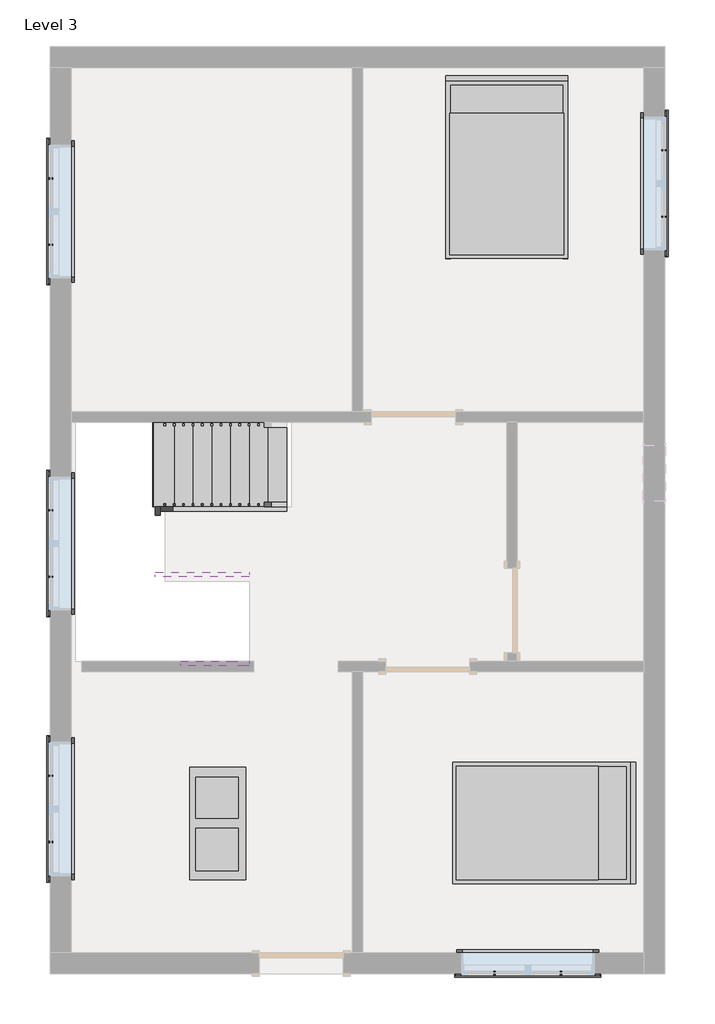
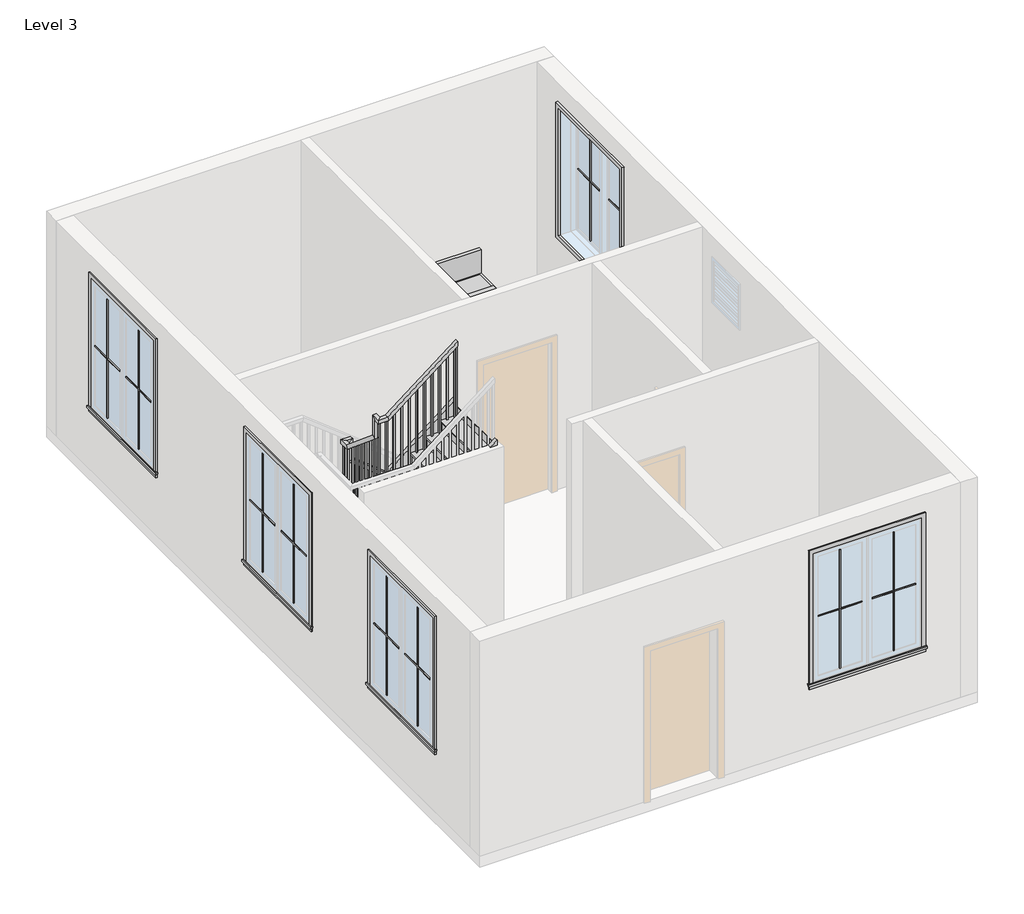
# One storey, part 2 of 2: 21 proxies, 5 members, 2 furniture elements, 1 railing, 1 stair flight.
"""IFC4 building model written with IfcOpenShell, lengths in millimetres."""

from ifc_helpers import new_model, si_unit, frame, origin, place, context, project, spatial, polyline, outline, extrude, faceted_brep, transform, mapped, element, save
from components import muntin_pattern_2x2_muntin_pattern_2x2_bff912c5, muntin_pattern_2x2_muntin_pattern_2x2_c2194282, trim_window_exterior_flat_with_sill_e04b3088, trim_window_interior_flat_picture_frame_2a7685fe, coffee_table_with_brass_mullions_11320_coffee_table_with_5962bef7, bed_17739_bed_17739_15c61121, stair_flight_32cec8f3

model = new_model("IFC4")

# Units and contexts
model_context = context("Model", 3, world=origin())
ifc_project = project(units=[si_unit("LENGTHUNIT", "METRE", prefix="MILLI")], contexts=[model_context])

# Site, building, storey
site = spatial("IfcSite", under=ifc_project)
building = spatial("IfcBuilding", under=site)
storey = spatial("IfcBuildingStorey", under=building, Name="Level 3", Elevation=3200.4)

# Proxies
placement = place(None, origin())
muntin_pattern_2x2_muntin_pattern_2x2_shape = muntin_pattern_2x2_muntin_pattern_2x2_bff912c5(model_context)
element("IfcBuildingElementProxy", 1, Name="Muntin Pattern_2x2 : Muntin Pattern_2x2", ObjectType="Muntin Pattern_2x2 : Muntin Pattern_2x2", at=placement, inside=storey, context=model_context, shape_type="MappedRepresentation", body=[
    mapped(muntin_pattern_2x2_muntin_pattern_2x2_shape, transform((-626.5715247, -5050.1430046, 4184.65), x_axis=(-1.0, 0.0, 0.0), y_axis=(0.0, -1.0, 0.0), z_axis=(0.0, 0.0, 1.0))),
])
element("IfcBuildingElementProxy", 2, Name="Muntin Pattern_2x2 : Muntin Pattern_2x2", ObjectType="Muntin Pattern_2x2 : Muntin Pattern_2x2", at=placement, inside=storey, context=model_context, shape_type="MappedRepresentation", body=[
    mapped(muntin_pattern_2x2_muntin_pattern_2x2_shape, transform((-6159.0090247, -3629.3305046, 4184.65), x_axis=(0.0, 1.0, 0.0), y_axis=(-1.0, 0.0, 0.0), z_axis=(0.0, 0.0, 1.0))),
])
element("IfcBuildingElementProxy", 3, Name="Muntin Pattern_2x2 : Muntin Pattern_2x2", ObjectType="Muntin Pattern_2x2 : Muntin Pattern_2x2", at=placement, inside=storey, context=model_context, shape_type="MappedRepresentation", body=[
    mapped(muntin_pattern_2x2_muntin_pattern_2x2_shape, transform((489.4409753, 3873.1944954, 4184.65), x_axis=(0.0, -1.0, 0.0), y_axis=(1.0, 0.0, 0.0), z_axis=(0.0, 0.0, 1.0))),
])
element("IfcBuildingElementProxy", 4, Name="Muntin Pattern_2x2 : Muntin Pattern_2x2", ObjectType="Muntin Pattern_2x2 : Muntin Pattern_2x2", at=placement, inside=storey, context=model_context, shape_type="MappedRepresentation", body=[
    mapped(muntin_pattern_2x2_muntin_pattern_2x2_shape, transform((-6159.0090247, 2847.6694954, 4184.65), x_axis=(0.0, 1.0, 0.0), y_axis=(-1.0, 0.0, 0.0), z_axis=(0.0, 0.0, 1.0))),
])
element("IfcBuildingElementProxy", 5, Name="Muntin Pattern_2x2 : Muntin Pattern_2x2", ObjectType="Muntin Pattern_2x2 : Muntin Pattern_2x2", at=placement, inside=storey, context=model_context, shape_type="MappedRepresentation", body=[
    mapped(muntin_pattern_2x2_muntin_pattern_2x2_shape, transform((-6159.0090247, -752.7805046, 4184.65), x_axis=(0.0, 1.0, 0.0), y_axis=(-1.0, 0.0, 0.0), z_axis=(0.0, 0.0, 1.0))),
])
muntin_pattern_2x2_muntin_pattern_2x2_2_shape = muntin_pattern_2x2_muntin_pattern_2x2_c2194282(model_context)
element("IfcBuildingElementProxy", 6, Name="Muntin Pattern_2x2 : Muntin Pattern_2x2", ObjectType="Muntin Pattern_2x2 : Muntin Pattern_2x2", at=placement, inside=storey, context=model_context, shape_type="MappedRepresentation", body=[
    mapped(muntin_pattern_2x2_muntin_pattern_2x2_2_shape, transform((-1347.2965247, -5050.1430046, 4184.65), x_axis=(1.0, 0.0, 0.0), y_axis=(0.0, 1.0, 0.0), z_axis=(0.0, 0.0, 1.0))),
])
element("IfcBuildingElementProxy", 7, Name="Muntin Pattern_2x2 : Muntin Pattern_2x2", ObjectType="Muntin Pattern_2x2 : Muntin Pattern_2x2", at=placement, inside=storey, context=model_context, shape_type="MappedRepresentation", body=[
    mapped(muntin_pattern_2x2_muntin_pattern_2x2_2_shape, transform((-6159.0090247, -2908.6055046, 4184.65), x_axis=(0.0, -1.0, 0.0), y_axis=(1.0, 0.0, 0.0), z_axis=(0.0, 0.0, 1.0))),
])
element("IfcBuildingElementProxy", 8, Name="Muntin Pattern_2x2 : Muntin Pattern_2x2", ObjectType="Muntin Pattern_2x2 : Muntin Pattern_2x2", at=placement, inside=storey, context=model_context, shape_type="MappedRepresentation", body=[
    mapped(muntin_pattern_2x2_muntin_pattern_2x2_2_shape, transform((489.4409753, 3152.4694954, 4184.65), x_axis=(0.0, 1.0, 0.0), y_axis=(-1.0, 0.0, 0.0), z_axis=(0.0, 0.0, 1.0))),
])
element("IfcBuildingElementProxy", 9, Name="Muntin Pattern_2x2 : Muntin Pattern_2x2", ObjectType="Muntin Pattern_2x2 : Muntin Pattern_2x2", at=placement, inside=storey, context=model_context, shape_type="MappedRepresentation", body=[
    mapped(muntin_pattern_2x2_muntin_pattern_2x2_2_shape, transform((-6159.0090247, 3568.3944954, 4184.65), x_axis=(0.0, -1.0, 0.0), y_axis=(1.0, 0.0, 0.0), z_axis=(0.0, 0.0, 1.0))),
])
element("IfcBuildingElementProxy", 10, Name="Muntin Pattern_2x2 : Muntin Pattern_2x2", ObjectType="Muntin Pattern_2x2 : Muntin Pattern_2x2", at=placement, inside=storey, context=model_context, shape_type="MappedRepresentation", body=[
    mapped(muntin_pattern_2x2_muntin_pattern_2x2_2_shape, transform((-6159.0090247, -32.0555046, 4184.65), x_axis=(0.0, -1.0, 0.0), y_axis=(1.0, 0.0, 0.0), z_axis=(0.0, 0.0, 1.0))),
])
trim_window_exterior_flat_with_sill_shape = trim_window_exterior_flat_with_sill_e04b3088(model_context)
element("IfcBuildingElementProxy", 11, Name="Trim-Window-Exterior-Flat : with Sill", ObjectType="Trim-Window-Exterior-Flat : with Sill", at=placement, inside=storey, context=model_context, shape_type="MappedRepresentation", body=[
    mapped(trim_window_exterior_flat_with_sill_shape, transform((-986.9340247, -5059.6680046, 5943.6), x_axis=(1.0, 0.0, 0.0), y_axis=(0.0, 0.0, 1.0), z_axis=(0.0, -1.0, 0.0))),
])
element("IfcBuildingElementProxy", 12, Name="Trim-Window-Exterior-Flat : with Sill", ObjectType="Trim-Window-Exterior-Flat : with Sill", at=placement, inside=storey, context=model_context, shape_type="MappedRepresentation", body=[
    mapped(trim_window_exterior_flat_with_sill_shape, transform((-6168.5340247, -3268.9680046, 5943.6), x_axis=(0.0, -1.0, 0.0), y_axis=(0.0, 0.0, 1.0), z_axis=(-1.0, 0.0, 0.0))),
])
element("IfcBuildingElementProxy", 13, Name="Trim-Window-Exterior-Flat : with Sill", ObjectType="Trim-Window-Exterior-Flat : with Sill", at=placement, inside=storey, context=model_context, shape_type="MappedRepresentation", body=[
    mapped(trim_window_exterior_flat_with_sill_shape, transform((498.9659753, 3512.8319954, 5943.6), x_axis=(0.0, 1.0, 0.0), y_axis=(0.0, 0.0, 1.0), z_axis=(1.0, 0.0, 0.0))),
])
element("IfcBuildingElementProxy", 14, Name="Trim-Window-Exterior-Flat : with Sill", ObjectType="Trim-Window-Exterior-Flat : with Sill", at=placement, inside=storey, context=model_context, shape_type="MappedRepresentation", body=[
    mapped(trim_window_exterior_flat_with_sill_shape, transform((-6168.5340247, 3208.0319954, 5943.6), x_axis=(0.0, -1.0, 0.0), y_axis=(0.0, 0.0, 1.0), z_axis=(-1.0, 0.0, 0.0))),
])
element("IfcBuildingElementProxy", 15, Name="Trim-Window-Exterior-Flat : with Sill", ObjectType="Trim-Window-Exterior-Flat : with Sill", at=placement, inside=storey, context=model_context, shape_type="MappedRepresentation", body=[
    mapped(trim_window_exterior_flat_with_sill_shape, transform((-6168.5340247, -392.4180046, 5943.6), x_axis=(0.0, -1.0, 0.0), y_axis=(0.0, 0.0, 1.0), z_axis=(-1.0, 0.0, 0.0))),
])
trim_window_interior_flat_picture_frame_shape = trim_window_interior_flat_picture_frame_2a7685fe(model_context)
element("IfcBuildingElementProxy", 16, Name="Trim-Window-Interior-Flat : Picture Frame", ObjectType="Trim-Window-Interior-Flat : Picture Frame", at=placement, inside=storey, context=model_context, shape_type="MappedRepresentation", body=[
    mapped(trim_window_interior_flat_picture_frame_shape, transform((-986.9340247, -4831.0680046, 5943.6), x_axis=(-1.0, 0.0, 0.0), y_axis=(0.0, 0.0, 1.0), z_axis=(0.0, 1.0, 0.0))),
])
element("IfcBuildingElementProxy", 17, Name="Trim-Window-Interior-Flat : Picture Frame", ObjectType="Trim-Window-Interior-Flat : Picture Frame", at=placement, inside=storey, context=model_context, shape_type="MappedRepresentation", body=[
    mapped(trim_window_interior_flat_picture_frame_shape, transform((-5939.9340247, -3268.9680046, 5943.6), x_axis=(0.0, 1.0, 0.0), y_axis=(0.0, 0.0, 1.0), z_axis=(1.0, 0.0, 0.0))),
])
element("IfcBuildingElementProxy", 18, Name="Trim-Window-Interior-Flat : Picture Frame", ObjectType="Trim-Window-Interior-Flat : Picture Frame", at=placement, inside=storey, context=model_context, shape_type="MappedRepresentation", body=[
    mapped(trim_window_interior_flat_picture_frame_shape, transform((270.3659753, 3512.8319954, 5943.6), x_axis=(0.0, -1.0, 0.0), y_axis=(0.0, 0.0, 1.0), z_axis=(-1.0, 0.0, 0.0))),
])
element("IfcBuildingElementProxy", 19, Name="Trim-Window-Interior-Flat : Picture Frame", ObjectType="Trim-Window-Interior-Flat : Picture Frame", at=placement, inside=storey, context=model_context, shape_type="MappedRepresentation", body=[
    mapped(trim_window_interior_flat_picture_frame_shape, transform((-5939.9340247, 3208.0319954, 5943.6), x_axis=(0.0, 1.0, 0.0), y_axis=(0.0, 0.0, 1.0), z_axis=(1.0, 0.0, 0.0))),
])
element("IfcBuildingElementProxy", 20, Name="Trim-Window-Interior-Flat : Picture Frame", ObjectType="Trim-Window-Interior-Flat : Picture Frame", at=placement, inside=storey, context=model_context, shape_type="MappedRepresentation", body=[
    mapped(trim_window_interior_flat_picture_frame_shape, transform((-5939.9340247, -392.4180046, 5943.6), x_axis=(0.0, 1.0, 0.0), y_axis=(0.0, 0.0, 1.0), z_axis=(1.0, 0.0, 0.0))),
])
coffee_table_with_brass_mullions_11320_coffee_table_with_shape = coffee_table_with_brass_mullions_11320_coffee_table_with_5962bef7(model_context)
element("IfcBuildingElementProxy", 21, Name="coffee_table_with_brass_mullions_11320 : coffee_table_with_brass_mullions_11320", ObjectType="coffee_table_with_brass_mullions_11320 : coffee_table_with_brass_mullions_11320", at=placement, inside=storey, context=model_context, shape_type="MappedRepresentation", body=[
    mapped(coffee_table_with_brass_mullions_11320_coffee_table_with_shape, transform((-3920.6340247, -2792.7180046, 3200.4), x_axis=(0.0, 1.0, 0.0), y_axis=(-1.0, 0.0, 0.0), z_axis=(0.0, 0.0, 1.0))),
])

# Furniture
bed_17739_bed_17739_shape = bed_17739_bed_17739_15c61121(model_context)
element("IfcFurniture", 22, ObjectType="Bed_17739 : Bed_17739", at=placement, inside=storey, context=model_context, shape_type="MappedRepresentation", body=[
    mapped(bed_17739_bed_17739_shape, transform((-1215.5340247, 3665.2319954, 3200.4), x_axis=(1.0, 0.0, 0.0), y_axis=(0.0, 1.0, 0.0), z_axis=(0.0, 0.0, 1.0))),
])
element("IfcFurniture", 23, ObjectType="Bed_17739 : Bed_17739", at=placement, inside=storey, context=model_context, shape_type="MappedRepresentation", body=[
    mapped(bed_17739_bed_17739_shape, transform((-834.5340247, -3421.3680046, 3200.4), x_axis=(0.0, -1.0, 0.0), y_axis=(1.0, 0.0, 0.0), z_axis=(0.0, 0.0, 1.0))),
])

# Members
element("IfcMember", 24, ObjectType="Stringer - 2\" Width", at=placement, inside=storey, context=model_context, shape_type="SweptSolid", body=[
    extrude(outline(polyline([(3200.4, -3603.1340247), (3431.9686588, -3603.1340247), (4514.8107641, -4974.7340247), (4126.4725136, -4974.7340247), (3200.4, -3801.7088408), (3200.4, -3603.1340247)])), frame((0.0, -43.1680046, 0.0), z_axis=(0.0, 1.0, 0.0), x_axis=(0.0, 0.0, 1.0)), (0.0, 0.0, 1.0), 50.8),
])
element("IfcMember", 25, ObjectType="Stringer - 2\" Width", at=placement, inside=storey, context=model_context, shape_type="SweptSolid", body=[
    extrude(outline(polyline([(7.6319954, 4721.6930346), (7.6319954, 4323.2154064), (-703.5680046, 4922.1206696), (-703.5680046, 5320.5982978), (7.6319954, 4721.6930346)])), frame((-5025.5340247, 0.0, 0.0), z_axis=(1.0, 0.0, 0.0), x_axis=(0.0, 1.0, 0.0)), (0.0, 0.0, 1.0), 50.8),
])
element("IfcMember", 26, ObjectType="Stringer - 2\" Width", at=placement, inside=storey, context=model_context, shape_type="SweptSolid", body=[
    extrude(outline(polyline([(5517.442343, -5025.5340247), (5129.1040926, -5025.5340247), (5931.2093557, -4009.5340247), (6319.5476062, -4009.5340247), (5517.442343, -5025.5340247)])), frame((0.0, -754.3680046, 0.0), z_axis=(0.0, 1.0, 0.0), x_axis=(0.0, 0.0, 1.0)), (0.0, 0.0, 1.0), 50.8),
])
element("IfcMember", 27, ObjectType="Stringer - 2\" Width", at=placement, inside=storey, context=model_context, shape_type="SweptSolid", body=[
    extrude(outline(polyline([(3200.4, -3603.1340247), (3431.9686588, -3603.1340247), (3951.671982, -4261.4249007), (3951.671982, -4753.3200179), (3200.4, -3801.7088408), (3200.4, -3603.1340247)])), frame((0.0, 922.0319954, 0.0), z_axis=(0.0, 1.0, 0.0), x_axis=(0.0, 0.0, 1.0)), (0.0, 0.0, 1.0), 50.8),
])
element("IfcMember", 28, ObjectType="Stringer - 2\" Width", at=placement, inside=storey, context=model_context, shape_type="SweptSolid", body=[
    extrude(outline(polyline([(5734.9206696, -4258.1663605), (5931.2093557, -4009.5340247), (6319.5476062, -4009.5340247), (5734.9206696, -4750.0614777), (5734.9206696, -4258.1663605)])), frame((0.0, -1719.5680046, 0.0), z_axis=(0.0, 1.0, 0.0), x_axis=(0.0, 0.0, 1.0)), (0.0, 0.0, 1.0), 50.8),
])

# Railing
element("IfcRailing", 29, ObjectType="Handrail - Rectangular", at=placement, inside=storey, context=model_context, shape_type="SolidModel", body=[
    faceted_brep([(-3603.1340247, 7.6319954, 4275.2210526), (-3603.1340247, 7.6319954, 4210.4980109), (-3603.1340247, 58.4319954, 4210.4980109), (-3603.1340247, 58.4319954, 4275.2210526), (-4949.3340247, 7.6319954, 5338.0105263), (-5000.1340247, 7.6319954, 5313.3927477), (-5000.1340247, 58.4319954, 5313.3927477), (-4949.3340247, 58.4319954, 5338.0105263), (-4949.3340247, 7.6319954, 5622.7578947), (-5000.1340247, 7.6319954, 5571.9578947), (-5000.1340247, 58.4319954, 5571.9578947), (-4949.3340247, 58.4319954, 5622.7578947), (-5025.5340247, 7.6319954, 5622.7578947), (-5025.5340247, 7.6319954, 5571.9578947), (-5076.3340247, 58.4319954, 5571.9578947), (-5076.3340247, 58.4319954, 5622.7578947), (-5025.5340247, -68.5680046, 5622.7578947), (-5025.5340247, -87.1083685, 5571.9578947), (-5076.3340247, -87.1083685, 5571.9578947), (-5076.3340247, -68.5680046, 5622.7578947), (-5025.5340247, -678.1680046, 6136.1052632), (-5025.5340247, -728.9680046, 6112.4712725), (-5076.3340247, -728.9680046, 6112.4712725), (-5076.3340247, -678.1680046, 6136.1052632), (-5025.5340247, -678.1680046, 6420.8526316), (-5025.5340247, -728.9680046, 6370.0526316), (-5076.3340247, -728.9680046, 6370.0526316), (-5076.3340247, -678.1680046, 6420.8526316), (-5025.5340247, -754.3680046, 6420.8526316), (-5025.5340247, -754.3680046, 6370.0526316), (-5076.3340247, -805.1680046, 6370.0526316), (-5076.3340247, -805.1680046, 6420.8526316), (-4949.3340247, -754.3680046, 6420.8526316), (-4931.6981718, -754.3680046, 6370.0526316), (-4931.6981718, -805.1680046, 6370.0526316), (-4949.3340247, -805.1680046, 6420.8526316), (-4009.5340247, -754.3680046, 7162.8), (-4009.5340247, -805.1680046, 7162.8), (-4009.5340247, -805.1680046, 7098.0769583), (-4009.5340247, -754.3680046, 7098.0769583)], [[[0, 1, 2, 3]], [[1, 0, 4, 5]], [[2, 1, 5, 6]], [[3, 2, 6, 7]], [[0, 3, 7, 4]], [[5, 4, 8, 9]], [[6, 5, 9, 10]], [[7, 6, 10, 11]], [[4, 7, 11, 8]], [[9, 8, 12, 13]], [[10, 9, 13, 14]], [[11, 10, 14, 15]], [[8, 11, 15, 12]], [[13, 12, 16, 17]], [[14, 13, 17, 18]], [[15, 14, 18, 19]], [[12, 15, 19, 16]], [[17, 16, 20, 21]], [[18, 17, 21, 22]], [[19, 18, 22, 23]], [[16, 19, 23, 20]], [[21, 20, 24, 25]], [[22, 21, 25, 26]], [[23, 22, 26, 27]], [[20, 23, 27, 24]], [[25, 24, 28, 29]], [[26, 25, 29, 30]], [[27, 26, 30, 31]], [[24, 27, 31, 28]], [[29, 28, 32, 33]], [[30, 29, 33, 34]], [[31, 30, 34, 35]], [[28, 31, 35, 32]], [[36, 37, 38, 39]], [[33, 32, 36, 39]], [[34, 33, 39, 38]], [[35, 34, 38, 37]], [[32, 35, 37, 36]]]),
    extrude(outline(polyline([(7070.5045898, -4044.4590247), (6087.9789474, -4044.4590247), (6087.9789474, -4025.4090247), (7085.5440635, -4025.4090247), (7070.5045898, -4044.4590247)])), frame((0.0, -789.2930046, 0.0), z_axis=(0.0, 1.0, 0.0), x_axis=(0.0, 0.0, 1.0)), (0.0, 0.0, 1.0), 19.05),
    extrude(outline(polyline([(6990.2940635, -4146.0590247), (6087.9789474, -4146.0590247), (6087.9789474, -4127.0090247), (7005.3335372, -4127.0090247), (6990.2940635, -4146.0590247)])), frame((0.0, -789.2930046, 0.0), z_axis=(0.0, 1.0, 0.0), x_axis=(0.0, 0.0, 1.0)), (0.0, 0.0, 1.0), 19.05),
    extrude(outline(polyline([(6910.0835372, -4247.6590247), (5927.5578947, -4247.6590247), (5927.5578947, -4228.6090247), (6925.1230109, -4228.6090247), (6910.0835372, -4247.6590247)])), frame((0.0, -789.2930046, 0.0), z_axis=(0.0, 1.0, 0.0), x_axis=(0.0, 0.0, 1.0)), (0.0, 0.0, 1.0), 19.05),
    extrude(outline(polyline([(6829.8730109, -4349.2590247), (5927.5578947, -4349.2590247), (5927.5578947, -4330.2090247), (6844.9124846, -4330.2090247), (6829.8730109, -4349.2590247)])), frame((0.0, -789.2930046, 0.0), z_axis=(0.0, 1.0, 0.0), x_axis=(0.0, 0.0, 1.0)), (0.0, 0.0, 1.0), 19.05),
    extrude(outline(polyline([(6749.6624846, -4450.8590247), (5767.1368421, -4450.8590247), (5767.1368421, -4431.8090247), (6764.7019583, -4431.8090247), (6749.6624846, -4450.8590247)])), frame((0.0, -789.2930046, 0.0), z_axis=(0.0, 1.0, 0.0), x_axis=(0.0, 0.0, 1.0)), (0.0, 0.0, 1.0), 19.05),
    extrude(outline(polyline([(6669.4519583, -4552.4590247), (5767.1368421, -4552.4590247), (5767.1368421, -4533.4090247), (6684.4914319, -4533.4090247), (6669.4519583, -4552.4590247)])), frame((0.0, -789.2930046, 0.0), z_axis=(0.0, 1.0, 0.0), x_axis=(0.0, 0.0, 1.0)), (0.0, 0.0, 1.0), 19.05),
    extrude(outline(polyline([(6589.2414319, -4654.0590247), (5606.7157895, -4654.0590247), (5606.7157895, -4635.0090247), (6604.2809056, -4635.0090247), (6589.2414319, -4654.0590247)])), frame((0.0, -789.2930046, 0.0), z_axis=(0.0, 1.0, 0.0), x_axis=(0.0, 0.0, 1.0)), (0.0, 0.0, 1.0), 19.05),
    extrude(outline(polyline([(6509.0309056, -4755.6590247), (5606.7157895, -4755.6590247), (5606.7157895, -4736.6090247), (6524.0703793, -4736.6090247), (6509.0309056, -4755.6590247)])), frame((0.0, -789.2930046, 0.0), z_axis=(0.0, 1.0, 0.0), x_axis=(0.0, 0.0, 1.0)), (0.0, 0.0, 1.0), 19.05),
    extrude(outline(polyline([(6428.8203793, -4857.2590247), (5446.2947368, -4857.2590247), (5446.2947368, -4838.2090247), (6443.859853, -4838.2090247), (6428.8203793, -4857.2590247)])), frame((0.0, -789.2930046, 0.0), z_axis=(0.0, 1.0, 0.0), x_axis=(0.0, 0.0, 1.0)), (0.0, 0.0, 1.0), 19.05),
    extrude(outline(polyline([(6348.609853, -4958.8590247), (5446.2947368, -4958.8590247), (5446.2947368, -4939.8090247), (6363.6493267, -4939.8090247), (6348.609853, -4958.8590247)])), frame((0.0, -789.2930046, 0.0), z_axis=(0.0, 1.0, 0.0), x_axis=(0.0, 0.0, 1.0)), (0.0, 0.0, 1.0), 19.05),
    extrude(outline(polyline([(-668.6430046, 6061.6712725), (-668.6430046, 5125.4526316), (-687.6930046, 5125.4526316), (-687.6930046, 6077.7133778), (-668.6430046, 6061.6712725)])), frame((-5060.4590247, 0.0, 0.0), z_axis=(1.0, 0.0, 0.0), x_axis=(0.0, 1.0, 0.0)), (0.0, 0.0, 1.0), 19.05),
    extrude(outline(polyline([(-567.0430046, 5976.1133778), (-567.0430046, 5125.4526316), (-586.0930046, 5125.4526316), (-586.0930046, 5992.155483), (-567.0430046, 5976.1133778)])), frame((-5060.4590247, 0.0, 0.0), z_axis=(1.0, 0.0, 0.0), x_axis=(0.0, 1.0, 0.0)), (0.0, 0.0, 1.0), 19.05),
    extrude(outline(polyline([(-465.4430046, 5890.555483), (-465.4430046, 4965.0315789), (-484.4930046, 4965.0315789), (-484.4930046, 5906.5975883), (-465.4430046, 5890.555483)])), frame((-5060.4590247, 0.0, 0.0), z_axis=(1.0, 0.0, 0.0), x_axis=(0.0, 1.0, 0.0)), (0.0, 0.0, 1.0), 19.05),
    extrude(outline(polyline([(-363.8430046, 5804.9975883), (-363.8430046, 4965.0315789), (-382.8930046, 4965.0315789), (-382.8930046, 5821.0396935), (-363.8430046, 5804.9975883)])), frame((-5060.4590247, 0.0, 0.0), z_axis=(1.0, 0.0, 0.0), x_axis=(0.0, 1.0, 0.0)), (0.0, 0.0, 1.0), 19.05),
    extrude(outline(polyline([(-262.2430046, 5719.4396935), (-262.2430046, 4804.6105263), (-281.2930046, 4804.6105263), (-281.2930046, 5735.4817988), (-262.2430046, 5719.4396935)])), frame((-5060.4590247, 0.0, 0.0), z_axis=(1.0, 0.0, 0.0), x_axis=(0.0, 1.0, 0.0)), (0.0, 0.0, 1.0), 19.05),
    extrude(outline(polyline([(-160.6430046, 5633.8817988), (-160.6430046, 4804.6105263), (-179.6930046, 4804.6105263), (-179.6930046, 5649.9239041), (-160.6430046, 5633.8817988)])), frame((-5060.4590247, 0.0, 0.0), z_axis=(1.0, 0.0, 0.0), x_axis=(0.0, 1.0, 0.0)), (0.0, 0.0, 1.0), 19.05),
    extrude(outline(polyline([(-59.0430046, 5548.3239041), (-59.0430046, 4644.1894737), (-78.0930046, 4644.1894737), (-78.0930046, 5564.3660093), (-59.0430046, 5548.3239041)])), frame((-5060.4590247, 0.0, 0.0), z_axis=(1.0, 0.0, 0.0), x_axis=(0.0, 1.0, 0.0)), (0.0, 0.0, 1.0), 19.05),
    extrude(outline(polyline([(-5016.0090247, 23.5069954), (-5035.0590247, 23.5069954), (-5035.0590247, 42.5569954), (-5016.0090247, 42.5569954), (-5016.0090247, 23.5069954)])), frame((0.0, 0.0, 4483.7684211), z_axis=(0.0, 0.0, 1.0), x_axis=(1.0, 0.0, 0.0)), (0.0, 0.0, 1.0), 1088.1894737),
    extrude(outline(polyline([(5260.7545898, -4933.4590247), (4323.3473684, -4933.4590247), (4323.3473684, -4914.4090247), (5245.7151161, -4914.4090247), (5260.7545898, -4933.4590247)])), frame((0.0, 23.5069954, 0.0), z_axis=(0.0, 1.0, 0.0), x_axis=(0.0, 0.0, 1.0)), (0.0, 0.0, 1.0), 19.05),
    extrude(outline(polyline([(5180.5440635, -4831.8590247), (4323.3473684, -4831.8590247), (4323.3473684, -4812.8090247), (5165.5045898, -4812.8090247), (5180.5440635, -4831.8590247)])), frame((0.0, 23.5069954, 0.0), z_axis=(0.0, 1.0, 0.0), x_axis=(0.0, 0.0, 1.0)), (0.0, 0.0, 1.0), 19.05),
    extrude(outline(polyline([(5100.3335372, -4730.2590247), (4162.9263158, -4730.2590247), (4162.9263158, -4711.2090247), (5085.2940635, -4711.2090247), (5100.3335372, -4730.2590247)])), frame((0.0, 23.5069954, 0.0), z_axis=(0.0, 1.0, 0.0), x_axis=(0.0, 0.0, 1.0)), (0.0, 0.0, 1.0), 19.05),
    extrude(outline(polyline([(5020.1230109, -4628.6590247), (4162.9263158, -4628.6590247), (4162.9263158, -4609.6090247), (5005.0835372, -4609.6090247), (5020.1230109, -4628.6590247)])), frame((0.0, 23.5069954, 0.0), z_axis=(0.0, 1.0, 0.0), x_axis=(0.0, 0.0, 1.0)), (0.0, 0.0, 1.0), 19.05),
    extrude(outline(polyline([(4939.9124846, -4527.0590247), (4002.5052632, -4527.0590247), (4002.5052632, -4508.0090247), (4924.8730109, -4508.0090247), (4939.9124846, -4527.0590247)])), frame((0.0, 23.5069954, 0.0), z_axis=(0.0, 1.0, 0.0), x_axis=(0.0, 0.0, 1.0)), (0.0, 0.0, 1.0), 19.05),
    extrude(outline(polyline([(4859.7019583, -4425.4590247), (4002.5052632, -4425.4590247), (4002.5052632, -4406.4090247), (4844.6624846, -4406.4090247), (4859.7019583, -4425.4590247)])), frame((0.0, 23.5069954, 0.0), z_axis=(0.0, 1.0, 0.0), x_axis=(0.0, 0.0, 1.0)), (0.0, 0.0, 1.0), 19.05),
    extrude(outline(polyline([(4779.4914319, -4323.8590247), (3842.0842105, -4323.8590247), (3842.0842105, -4304.8090247), (4764.4519583, -4304.8090247), (4779.4914319, -4323.8590247)])), frame((0.0, 23.5069954, 0.0), z_axis=(0.0, 1.0, 0.0), x_axis=(0.0, 0.0, 1.0)), (0.0, 0.0, 1.0), 19.05),
    extrude(outline(polyline([(4699.2809056, -4222.2590247), (3842.0842105, -4222.2590247), (3842.0842105, -4203.2090247), (4684.2414319, -4203.2090247), (4699.2809056, -4222.2590247)])), frame((0.0, 23.5069954, 0.0), z_axis=(0.0, 1.0, 0.0), x_axis=(0.0, 0.0, 1.0)), (0.0, 0.0, 1.0), 19.05),
    extrude(outline(polyline([(4619.0703793, -4120.6590247), (3681.6631579, -4120.6590247), (3681.6631579, -4101.6090247), (4604.0309056, -4101.6090247), (4619.0703793, -4120.6590247)])), frame((0.0, 23.5069954, 0.0), z_axis=(0.0, 1.0, 0.0), x_axis=(0.0, 0.0, 1.0)), (0.0, 0.0, 1.0), 19.05),
    extrude(outline(polyline([(4538.859853, -4019.0590247), (3681.6631579, -4019.0590247), (3681.6631579, -4000.0090247), (4523.8203793, -4000.0090247), (4538.859853, -4019.0590247)])), frame((0.0, 23.5069954, 0.0), z_axis=(0.0, 1.0, 0.0), x_axis=(0.0, 0.0, 1.0)), (0.0, 0.0, 1.0), 19.05),
    extrude(outline(polyline([(4458.6493267, -3917.4590247), (3521.2421053, -3917.4590247), (3521.2421053, -3898.4090247), (4443.609853, -3898.4090247), (4458.6493267, -3917.4590247)])), frame((0.0, 23.5069954, 0.0), z_axis=(0.0, 1.0, 0.0), x_axis=(0.0, 0.0, 1.0)), (0.0, 0.0, 1.0), 19.05),
    extrude(outline(polyline([(4378.4388004, -3815.8590247), (3521.2421053, -3815.8590247), (3521.2421053, -3796.8090247), (4363.3993267, -3796.8090247), (4378.4388004, -3815.8590247)])), frame((0.0, 23.5069954, 0.0), z_axis=(0.0, 1.0, 0.0), x_axis=(0.0, 0.0, 1.0)), (0.0, 0.0, 1.0), 19.05),
    extrude(outline(polyline([(4298.228274, -3714.2590247), (3360.8210526, -3714.2590247), (3360.8210526, -3695.2090247), (4283.1888004, -3695.2090247), (4298.228274, -3714.2590247)])), frame((0.0, 23.5069954, 0.0), z_axis=(0.0, 1.0, 0.0), x_axis=(0.0, 0.0, 1.0)), (0.0, 0.0, 1.0), 19.05),
    extrude(outline(polyline([(-5041.4090247, -770.2430046), (-5041.4090247, -789.2930046), (-5060.4590247, -789.2930046), (-5060.4590247, -770.2430046), (-5041.4090247, -770.2430046)])), frame((0.0, 0.0, 5285.8736842), z_axis=(0.0, 0.0, 1.0), x_axis=(1.0, 0.0, 0.0)), (0.0, 0.0, 1.0), 1084.1789474),
    extrude(outline(polyline([(-5041.4090247, 23.5069954), (-5060.4590247, 23.5069954), (-5060.4590247, 42.5569954), (-5041.4090247, 42.5569954), (-5041.4090247, 23.5069954)])), frame((0.0, 0.0, 4483.7684211), z_axis=(0.0, 0.0, 1.0), x_axis=(1.0, 0.0, 0.0)), (0.0, 0.0, 1.0), 1088.1894737),
    extrude(outline(polyline([(7083.0374846, -4028.5840247), (6087.9789474, -4028.5840247), (6087.9789474, -4009.5340247), (7098.0769583, -4009.5340247), (7083.0374846, -4028.5840247)])), frame((0.0, -789.2930046, 0.0), z_axis=(0.0, 1.0, 0.0), x_axis=(0.0, 0.0, 1.0)), (0.0, 0.0, 1.0), 19.05),
    extrude(outline(polyline([(4225.5374846, -3622.1840247), (3360.8210526, -3622.1840247), (3360.8210526, -3603.1340247), (4210.4980109, -3603.1340247), (4225.5374846, -3622.1840247)])), frame((0.0, 23.5069954, 0.0), z_axis=(0.0, 1.0, 0.0), x_axis=(0.0, 0.0, 1.0)), (0.0, 0.0, 1.0), 19.05),
])

# Stair flight
stair_flight_shape = stair_flight_32cec8f3(model_context)
element("IfcStairFlight", 30, ObjectType="2\" Tread 1\" Nosing 1/4\" Riser", at=placement, inside=storey, context=model_context, shape_type="MappedRepresentation", body=[
    mapped(stair_flight_shape, transform((0.0, 0.0, 0.0), x_axis=(1.0, 0.0, 0.0), y_axis=(0.0, 1.0, 0.0), z_axis=(0.0, 0.0, 1.0))),
])

save(model, "model.ifc")

# Revit data of these elements
# Type "Muntin Pattern_2x2 : Muntin Pattern_2x2"
#   Width [instance default] = 4' - 0"
#   Thickness = 0' - 0 1/2"
#   Height [instance default] = 4' - 0"
#   Distance = 0' - 0 3/4"
#   Interior Material [instance default] = none
#   Exterior Material [instance default] = none
#   Default Elevation = 0
# Type "Trim-Window-Exterior-Flat : with Sill"
#   Trim Width = 0' - 2 1/4"
#   Trim Thickness_Picture Frame = 0' - 1 1/4"
#   Trim Thickness_with Sill = 0' - 0 3/4"
#   Sill Thickness = 0' - 1 1/4"
#   Opening Width [instance default] = 2' - 0"
#   Opening Height [instance default] = 3' - 0"
#   Default Elevation = 4' - 0"
#   Sill = yes
#   Picture Frame = no
#   Trim Material [instance default] = none
# Type "Trim-Window-Interior-Flat : Picture Frame"
#   Trim Thickness_Picture Frame = 0' - 1 1/4"
#   Trim Width = 0' - 2 1/4"
#   Trim Thickness_with Sill = 0' - 0 3/4"
#   Sill Thickness = 0' - 1 1/4"
#   Opening Width [instance default] = 2' - 0"
#   Opening Height [instance default] = 3' - 0"
#   Default Elevation = 4' - 0"
#   Sill = no
#   Picture Frame = yes
#   Trim Material [instance default] = none
# Type "coffee_table_with_brass_mullions_11320 : coffee_table_with_brass_mullions_11320"
#   Default Elevation = 0
# Type "Bed_17739 : Bed_17739"
#   Default Elevation = 0
# Type "Handrail - Rectangular"
#   Assembly Code = "C2010400"
#   built-in parameter 1008612 = 0.0416667 (stored number, unit not read)
#   built-in parameter 1008611 = 0.0416667 (stored number, unit not read)
#   built-in parameter 1008609 = 0.333333 (stored number, unit not read)
#   built-in parameter 1008604 = 0.166667 (stored number, unit not read)
#   built-in parameter 1008603 = 0.166667 (stored number, unit not read)
#   Railing Height = 3' - 0"
#   built-in parameter 1008630 = 2
#   built-in parameter 1008610 = 2
#   built-in parameter 1008618 = Baluster - Square : 3/4"
# Elements 1, 2, 3, 4, 5, 6, 7, 8, 9, 10 (IfcBuildingElementProxy, "Muntin Pattern_2x2 : Muntin Pattern_2x2")
#   Width = 1' - 11 1/8"
#   Height = 5' - 6 1/2"
#   Interior Material = Wood - Stained
#   Exterior Material = Clad - White
#   Phase Created = New Construction
#   Materials on its faces: "Clad - White", "Wood - Stained"
# Elements 11, 12, 13, 14, 15 (IfcBuildingElementProxy, "Trim-Window-Exterior-Flat : with Sill")
#   Opening Width = 4' - 9"
#   Opening Height = 6' - 0"
#   Trim Material = Clad - White
#   Phase Created = New Construction
#   Materials on its faces: "Clad - White"
# Elements 16, 17, 18, 19, 20 (IfcBuildingElementProxy, "Trim-Window-Interior-Flat : Picture Frame")
#   Opening Width = 4' - 9"
#   Opening Height = 6' - 0"
#   Trim Material = Wood - Stained
#   Phase Created = New Construction
#   Materials on its faces: "Wood - Stained"
# Element 21 (IfcBuildingElementProxy, "coffee_table_with_brass_mullions_11320 : coffee_table_with_brass_mullions_11320")
#   Phase Created = New Construction
#   Materials on its faces: "Default Wall", "TABLE", "Glass", "Default"
# Elements 22, 23 (IfcFurniture, "Bed_17739 : Bed_17739")
#   Phase Created = New Construction
#   Materials on its faces: "legs", "sheets", "bed frame", "Blanket"
# Elements 24, 25, 26, 27, 28 (IfcMember, "Stringer - 2\" Width")
#   Phase Created = New Construction
# Element 29 (IfcRailing, "Handrail - Rectangular")
#   Phase Created = New Construction
#   Materials on its faces: "Oak Flooring"
# Element 30 (IfcStairFlight, "2\" Tread 1\" Nosing 1/4\" Riser")
#   Phase Created = New Construction
# Materials
#   "Clad - White": class "Wood", colour RGB 242 242 238, transparency 0, Cost = 0
#   "Wood - Stained": class "Wood", colour RGB 224 178 126, transparency 0, Cost = 0
#   "Default Wall": colour RGB 128 128 128, transparency 0, Cost = 0
#   "TABLE": class "Generic", colour RGB 120 120 120, transparency 0, Cost = 0
#   "Glass": class "Glass", colour RGB 0 128 192, transparency 0.75, Description = "Soda Lime Glass", Cost = 0
#   "Default": colour RGB 127 127 127, transparency 0, Cost = 0
#   "legs": colour RGB 90 73 37, transparency 0, Cost = 0
#   "sheets": colour RGB 200 195 176, transparency 0, Cost = 0
#   "bed frame": colour RGB 90 73 37, transparency 0, Cost = 0
#   "Blanket": class "System", colour RGB 59 0 1, transparency 0, Cost = 0
#   "Oak Flooring": class "Wood", colour RGB 216 169 114, transparency 0, Description = "Quercus Rubra", Cost = 0
